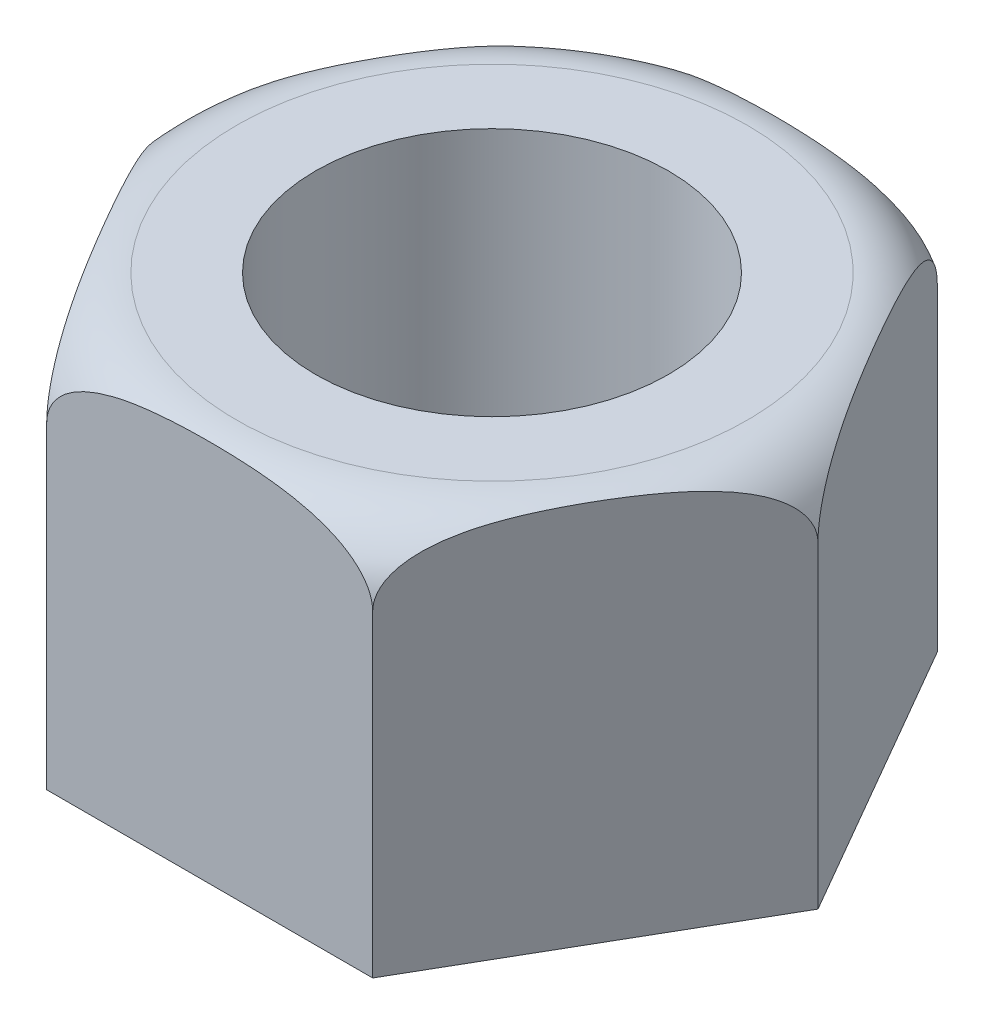
from build123d import *

# Parameters (mm, degrees)
HEX_BODY_16AF_X_11_DEPTH = 5.5
BORE_SKETCH_10_R         = 5
BORE_10_THROUGH_DEPTH    = 17.441816779


with BuildPart() as part:
    # Hex Profile 16AF Sketch → Hex Body 16AF x 11 (new, symmetric)
    with BuildSketch(Plane(origin=(0, 0, 0), x_dir=(1, 0, 0), z_dir=(0, 1, 0))):
        Polygon((9.237604307, 0), (4.618802154, 8), (-4.618802154, 8), (-9.237604307, 0), (-4.618802154, -8), (4.618802154, -8), align=None)
    extrude(amount=HEX_BODY_16AF_X_11_DEPTH, both=True)

    # Chamfer Profile Sketch → Face Chamfer 2mm (revolve, cut)
    with BuildSketch(Plane.XY, mode=Mode.PRIVATE) as face_chamfer_2mm_sk:
        with BuildLine():
            Line((9.237604307, 3.5), (9.237604307, -5.5))
            Line((9.237604307, -5.5), (12.102974232, -5.5))
            Line((12.102974232, -5.5), (12.102974232, 7.625857748))
            Line((12.102974232, 7.625857748), (4.618802154, 7.625857748))
            Line((4.618802154, 7.625857748), (4.618802154, 5.5))
            Line((4.618802154, 5.5), (7.237604307, 5.5))
            ThreePointArc((7.237604307, 5.5), (8.651817869, 4.914213562), (9.237604307, 3.5))
        make_face()
    revolve(face_chamfer_2mm_sk.sketch.rotate(Axis((0, 0, 0), (0, 1, 0)), 90), axis=Axis((0, 0, 0), (0, 1, 0)), mode=Mode.SUBTRACT)

    # Bore Sketch Ø10 → Bore Ø10 Through (cut, through all)
    with BuildSketch(Plane(origin=(0, 5.5, 0), x_dir=(1, 0, 0), z_dir=(0, 1, 0))):
        with Locations(Location((0, 0, 0), (0, 0, 270))):
            Circle(BORE_SKETCH_10_R)
    extrude(amount=-BORE_10_THROUGH_DEPTH, mode=Mode.SUBTRACT)


solid = part.part
